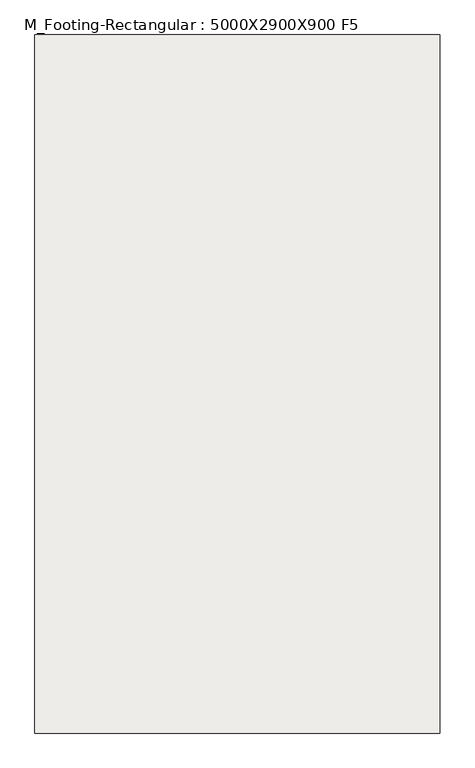
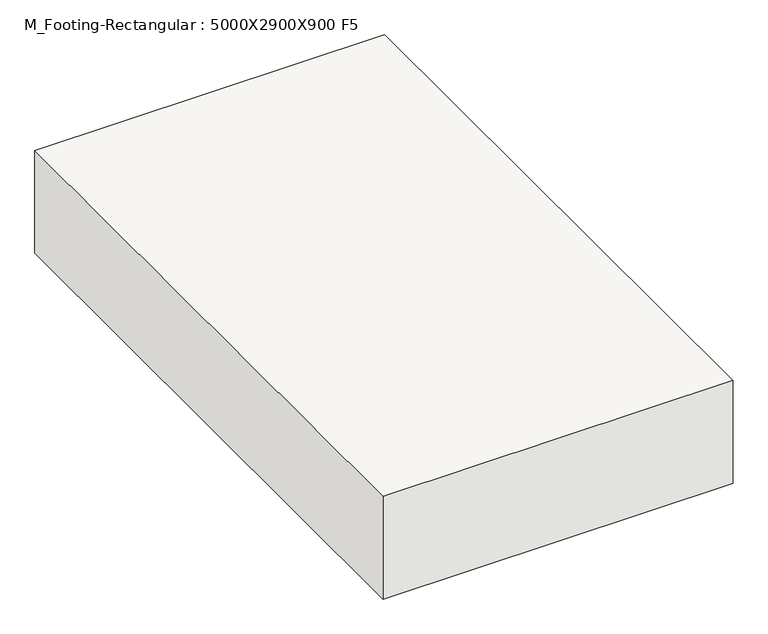
"""IFC4 building model written with IfcOpenShell, lengths in millimetres: slab geometry, M_Footing-Rectangular : 5000X2900X900 F5."""

from ifc_helpers import new_model, si_unit, frame, origin, place, context, project, spatial, polyline, outline, extrude, source, transform, mapped, element, save


def m_footing_rectangular_5000x2900x900_f5_2a8e231f(model_context):
    return source(origin(), model_context, "Body", "SweptSolid", [
        extrude(outline(polyline([(1450.0, 2500.0), (1450.0, -2500.0), (-1450.0, -2500.0), (-1450.0, 2500.0), (1450.0, 2500.0)])), frame((0.0, 0.0, -900.0), z_axis=(0.0, 0.0, 1.0), x_axis=(1.0, 0.0, 0.0)), (0.0, 0.0, 1.0), 900.0),
    ])


if __name__ == "__main__":
    model = new_model("IFC4")
    model_context = context("Model", 3, world=origin())
    ifc_project = project(units=[si_unit("LENGTHUNIT", "METRE", prefix="MILLI")], contexts=[model_context])
    site = spatial("IfcSite", under=ifc_project)
    building = spatial("IfcBuilding", under=site)
    placement = place(None, origin())
    m_footing_rectangular_5000x2900x900_f5_shape = m_footing_rectangular_5000x2900x900_f5_2a8e231f(model_context)
    element("IfcSlab", 1, ObjectType="M_Footing-Rectangular : 5000X2900X900 F5", at=placement, inside=building, context=model_context, shape_type="MappedRepresentation", body=[
        mapped(m_footing_rectangular_5000x2900x900_f5_shape, transform((0.0, 0.0, 0.0), x_axis=(1.0, 0.0, 0.0), y_axis=(0.0, 1.0, 0.0), z_axis=(0.0, 0.0, 1.0))),
    ])
    save(model, "model.ifc")

# Revit data of these elements
# Type "M_Footing-Rectangular : 5000X2900X900 F5"
#   Width = 2900 mm
#   Length = 5000 mm
#   Foundation Thickness = 900 mm
#   Structural Material [instance default] = Concrete, Cast-in-Place gray
#   Assembly Code = ""
# Element 1 (IfcSlab, "M_Footing-Rectangular : 5000X2900X900 F5")
#   Structural Material = Concrete, Cast In Situ
#   Materials on its faces: "Concrete, Cast In Situ"
# Materials
#   "Concrete, Cast-in-Place gray": class "Concrete", colour RGB 192 192 192, transparency 0, Description = "Cast-in-place concrete", Cost = 0
#   "Concrete, Cast In Situ": class "Concrete", colour RGB 192 192 192, transparency 0, Description = "physical material", Cost = 0
